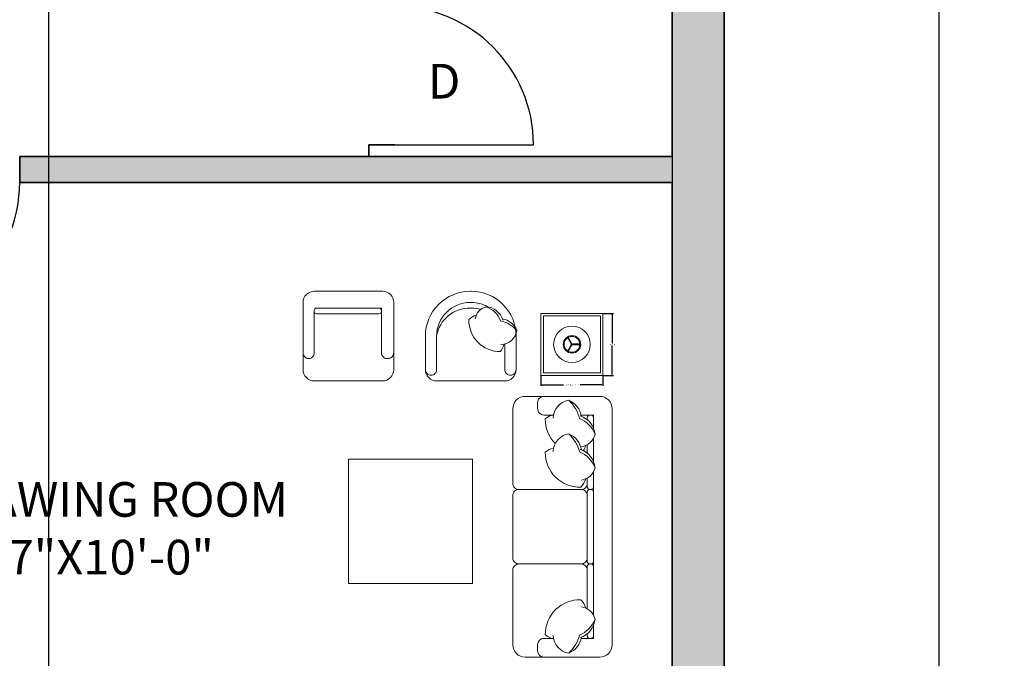
# Model space of a CAD drawing. Units: inches. Extents: x -5 to 330, y -522 to 40.
# Tile 19 of 23: x 159 to 330, y -380 to -269. Entities that reach past the tile are written whole.
import ezdxf

# ---------------------------------------------------------------- set-up
doc = ezdxf.new("R2010")
doc.units = ezdxf.units.IN
doc.header["$MEASUREMENT"] = 0
for name, color, linetype, lineweight in [('A-ANNO-DIMS', 2, 'Continuous', 18), ('A-ANNO-TEXT', 7, 'Continuous', 18), ('A-AREA-IDEN', 7, 'Continuous', 25), ('A-DOOR', 4, 'Continuous', 25), ('A-FURN', 8, 'Continuous', 18), ('A-WALL', 7, 'Continuous', 35)]:
    doc.layers.add(name, color=color, linetype=linetype, lineweight=lineweight)
doc.layers.add('A-WALL-PATT', color=18, linetype='Continuous', lineweight=13, true_color=0x000000)
doc.styles.get("Standard").update_dxf_attribs({"font": 'arial.ttf'})
doc.dimstyles.get("Standard").update_dxf_attribs({"dimtxt": 0.18, "dimasz": 0.18, "dimexe": 0.18, "dimexo": 0.0625, "dimgap": 0.09, "dimtad": 0, "dimtih": 1, "dimtoh": 1, "dimdec": 0, "dimzin": 0, "dimdsep": 46, "dimlunit": 3, "dimtxsty": 'Standard', "dimcen": 0.09, "dimadec": 0, "dimazin": 0, "dimtfac": 1, "dimtdec": 0, "dimtofl": 0, "dimtmove": 0, "dimatfit": 3, "dimfxl": 1, "dimtolj": 1, "dimtzin": 0, "dimarcsym": 0})

# ---------------------------------------------------------------- blocks, each defined once
blk = doc.blocks.new('*D6')
at = {"layer": 'A-ANNO-DIMS', "color": 0, "lineweight": -2, "transparency": 16777216}
for p, q in [((281.07, 12.36), (318.43, 12.36)), ((318.25, 12.18), (318.25, -238.29)), ((318.25, -494.96), (318.25, -244.5)), ((281.07, -495.14), (318.43, -495.14))]:
    blk.add_line(p, q, dxfattribs=at)
at = {"layer": 'A-ANNO-DIMS', "color": 0, "transparency": 16777216}
for points in [[(318.22, 12.18), (318.28, 12.18), (318.25, 12.36)], [(318.22, -494.96), (318.28, -494.96), (318.25, -495.14)]]:
    blk.add_solid(points, dxfattribs=at)
at = {"layer": 'Defpoints', "color": 0, "transparency": 16777216}
for p in [(281.01, 12.36), (281.01, -495.14), (318.25, -495.14)]:
    blk.add_point(p, dxfattribs=at)
at = {"layer": 'A-ANNO-DIMS', "color": 0, "transparency": 16777216, "insert": (318.25, -241.39), "char_height": 6, "attachment_point": 5}
blk.add_mtext('\\A1;42\'-4"', dxfattribs=at)
blk = doc.blocks.new('DOOR-24IN-SWING')
blk.add_line((24, 0), (24, 24))
blk.add_arc((24, 0), 24, 90, 180)
blk = doc.blocks.new('END-TABLE-SQUARE')
for p, q in [((5.32, 5.34), (4.56, 6.66)), ((5.32, 5.41), (4.56, 4.1)), ((5.44, 5.41), (4.68, 6.72)), ((5.44, 5.34), (4.68, 4.03)), ((5.38, 5.44), (6.89, 5.44)), ((5.38, 5.31), (6.89, 5.31))]:
    blk.add_line(p, q)
at = {"ltscale": 0.03}
blk.add_lwpolyline([(0, 0), (0, 10.75), (10.75, 10.75), (10.75, 0)], close=True, dxfattribs=at)
blk.add_lwpolyline([(0.43, 10.32), (0.43, 0.43), (10.32, 0.43), (10.32, 10.32)], close=True)
for radius in [3.17, 1.52, 1.36]:
    blk.add_circle((5.38, 5.38), radius)
blk = doc.blocks.new('*D27')
at = {"layer": 'A-ANNO-DIMS', "color": 0, "lineweight": -2, "transparency": 16777216}
for p, q in [((249.29, -330.63), (249.29, -332.36)), ((260.04, -330.63), (260.04, -332.36)), ((249.47, -332.18), (253.23, -332.18)), ((259.86, -332.18), (256.1, -332.18))]:
    blk.add_line(p, q, dxfattribs=at)
at = {"layer": 'A-ANNO-DIMS', "color": 0, "transparency": 16777216}
for points in [[(249.47, -332.15), (249.47, -332.21), (249.29, -332.18)], [(259.86, -332.15), (259.86, -332.21), (260.04, -332.18)]]:
    blk.add_solid(points, dxfattribs=at)
at = {"layer": 'Defpoints', "color": 0, "transparency": 16777216}
for p in [(249.29, -330.56), (260.04, -330.56), (260.04, -332.18)]:
    blk.add_point(p, dxfattribs=at)
at = {"layer": 'A-ANNO-DIMS', "color": 0, "transparency": 16777216, "insert": (254.67, -332.18), "char_height": 0.18, "attachment_point": 5}
blk.add_mtext('\\A1;END TABLE 0\'-11" TYP.', dxfattribs=at)
blk = doc.blocks.new('*D28')
at = {"layer": 'A-ANNO-DIMS', "color": 0, "lineweight": -2, "transparency": 16777216}
for p, q in [((260.11, -319.81), (261.84, -319.81)), ((261.66, -319.99), (261.66, -325)), ((261.66, -330.38), (261.66, -325.37)), ((260.11, -330.56), (261.84, -330.56))]:
    blk.add_line(p, q, dxfattribs=at)
at = {"layer": 'A-ANNO-DIMS', "color": 0, "transparency": 16777216}
for points in [[(261.63, -319.99), (261.69, -319.99), (261.66, -319.81)], [(261.63, -330.38), (261.69, -330.38), (261.66, -330.56)]]:
    blk.add_solid(points, dxfattribs=at)
at = {"layer": 'Defpoints', "color": 0, "transparency": 16777216}
for p in [(260.04, -319.81), (261.66, -319.81), (260.04, -330.56)]:
    blk.add_point(p, dxfattribs=at)
at = {"layer": 'A-ANNO-DIMS', "color": 0, "transparency": 16777216, "insert": (261.66, -325.19), "char_height": 0.18, "attachment_point": 5}
blk.add_mtext('\\A1;0\'-11" TYP.', dxfattribs=at)
blk = doc.blocks.new('*D37')
at = {"layer": 'A-ANNO-DIMS', "color": 0, "lineweight": -2, "transparency": 16777216}
for p, q in [((164.01, -53.21), (164.01, -522.31)), ((272.01, -53.21), (272.01, -522.31)), ((164.19, -522.13), (217.68, -522.13)), ((271.83, -522.13), (218.34, -522.13))]:
    blk.add_line(p, q, dxfattribs=at)
at = {"layer": 'A-ANNO-DIMS', "color": 0, "transparency": 16777216}
for points in [[(164.19, -522.1), (164.19, -522.16), (164.01, -522.13)], [(271.83, -522.1), (271.83, -522.16), (272.01, -522.13)]]:
    blk.add_solid(points, dxfattribs=at)
at = {"layer": 'Defpoints', "color": 0, "transparency": 16777216}
for p in [(164.01, -53.14), (272.01, -53.14), (272.01, -522.13)]:
    blk.add_point(p, dxfattribs=at)
at = {"layer": 'A-ANNO-DIMS', "color": 0, "transparency": 16777216, "insert": (218.01, -522.13), "char_height": 0.18, "attachment_point": 5}
blk.add_mtext('\\A1;9\'-0"', dxfattribs=at)

msp = doc.modelspace()

# ---------------------------------------------------------------- hatches: boundary and pattern name
at = {"layer": 'A-WALL-PATT'}
h = msp.add_hatch(color=256, dxfattribs=at)
h.dxf.hatch_style = 1
h.paths.add_polyline_path([(164.01, -44.15), (159.51, -44.15), (159.51, -153.14), (164.01, -153.14)], flags=17)
h.paths.add_polyline_path([(224.01, -188.14), (272.01, -188.14), (272.01, -218.14), (260.01, -218.14), (260.01, -222.64), (272.01, -222.64), (272.01, -292.64), (159.01, -292.64), (159.01, -297.14), (272.01, -297.14), (272.01, -417.14), (245.51, -417.14), (245.51, -426.14), (272.01, -426.14), (272.01, -495.14), (281.01, -495.14), (281.01, 12.36), (23.51, 12.36), (23.51, -426.14), (62.92, -426.14), (62.92, -417.14), (32.51, -417.14), (32.51, -297.14), (48.13, -297.14), (48.13, -292.64), (32.51, -292.64), (32.51, -140.64), (133.51, -140.64), (133.51, -131.64), (32.51, -131.64), (32.51, 3.36), (159.51, 3.36), (164.01, 3.36), (220.01, 3.36), (224.51, 3.36), (272.01, 3.36), (272.01, -179.14), (159.51, -179.14), (159.51, -188.14), (219.51, -188.14), (219.51, -266.64), (224.01, -266.64), (224.01, -222.64), (236.01, -222.64), (236.01, -218.14), (224.01, -218.14)])
h.paths.add_polyline_path([(133.01, -292.64), (128.51, -292.64), (128.51, -297.14), (128.51, -417.14), (122.92, -417.14), (122.92, -426.14), (133.01, -426.14)], flags=17)
h.paths.add_polyline_path([(185.51, -417.14), (159.01, -417.14), (159.01, -426.14), (185.51, -426.14)], flags=17)
h.paths.add_polyline_path([(133.51, -140.64), (129.01, -140.64), (129.01, -246.64), (133.51, -246.64)], flags=17)
h.paths.add_polyline_path([(246.01, -48.64), (224.51, -48.64), (224.51, -27.63), (220.01, -27.63), (220.01, -48.64), (198.6, -48.64), (198.6, -53.14), (246.01, -53.14)], flags=17)

# ---------------------------------------------------------------- linework, layer by layer
at = {"layer": 'A-FURN', "ltscale": 0.03}
for points in [[(210.04, -315.99), (210.04, -315.99, 0.414214), (208.1, -317.93), (208.1, -329.57, 0.414214), (210.04, -331.51), (210.04, -331.51), (221.87, -331.51, 0.414214), (223.8, -329.57), (223.8, -317.93, 0.414214), (221.87, -315.99)], [(246.57, -379.35, -0.414214), (244.42, -377.2), (244.42, -364.3, -0.414214), (245.5, -363.22, -0.414214), (244.42, -362.15), (244.42, -351.4, -0.414214), (245.5, -350.32, -0.414214), (244.42, -349.24), (244.42, -336.34, -0.414214), (246.57, -334.19), (259.48, -334.19, -0.414214), (261.63, -336.34), (261.63, -377.2, -0.414214), (259.48, -379.35)]]:
    msp.add_lwpolyline(points, format="xyb", close=True, dxfattribs=at)
msp.add_lwpolyline([(237.14, -331.51), (231.23, -331.51, -0.414214), (229.29, -329.57), (229.29, -323.75, -0.414214), (237.04, -315.99), (237.14, -315.99), (237.24, -315.99, -0.414214), (244.99, -323.75), (244.99, -329.57, -0.414214), (243.05, -331.51), (237.14, -331.51)], format="xyb", dxfattribs=at)
at = {"layer": 'A-FURN'}
for points in [[(218.02, -318.9), (210.42, -318.9, 0.414214), (210.04, -319.29), (210.04, -319.49, 0.414214), (210.42, -319.87), (217.04, -319.87, 0.414214)], [(217.04, -319.87), (221.28, -319.87, 0.414214), (221.67, -319.49), (221.67, -319.29, 0.414214), (221.28, -318.9)], [(221.28, -318.9), (218.02, -318.9, 0.414214)], [(231.23, -323.75, -0.414214), (237.04, -317.93), (237.14, -317.93)], [(231.23, -323.75, -0.372719), (237.04, -318.9), (237.14, -318.9)], [(240.12, -318.7, 0.130591), (237.24, -317.93), (237.14, -317.93)], [(238.89, -319.11, 0.072384), (237.24, -318.9), (237.14, -318.9)], [(242.71, -320.97, 0.306663), (239.82, -318.66, 0.30633), (237.93, -320.77, -0.872847)], [(245.15, -322.77, 0.14773), (242.32, -321.11, 0.213343), (239.82, -318.66, 0.178662)], [(210.04, -319.49), (210.04, -326.66, -0.414214), (209.07, -327.63), (209.07, -327.63, -0.414214), (208.1, -326.66)], [(242.86, -325.16, -0.165541), (242.26, -326.44, -0.425989), (236.82, -320.88, -0.121523), (238.11, -320.12, 7.115464)], [(242.37, -325.22, 0.356772), (245.15, -322.77, 0.249542), (242.63, -320.76, -9.61688)], [(231.23, -323.75), (231.23, -329.57, -0.414214), (230.26, -330.54), (230.26, -330.54, -0.414214), (229.29, -329.57)], [(223.8, -326.66, -0.414214), (222.83, -327.63), (222.64, -327.63, -0.414214), (221.67, -326.66), (221.67, -325.16)], [(243.05, -325.11), (243.05, -329.57, 0.414214), (244.02, -330.54), (244.02, -330.54, 0.414214), (244.99, -329.57)], [(251.47, -337.42), (249.8, -337.42, -0.414214), (248.72, -336.34), (248.72, -335.27, -0.414214), (249.8, -334.19)], [(251.4, -337.96, -0.356772), (254.11, -334.87, -0.249542), (256.34, -337.67, 9.61688)], [(254.11, -334.87, -0.14773), (255.96, -338.02, -0.213343), (258.67, -340.79, -0.178662)], [(251.47, -337.41, 0.165541), (250.04, -338.08, 0.200231), (251.78, -342.35, 0.121523)], [(256.11, -337.58, -0.306663), (258.67, -340.79, -0.30633), (256.33, -342.89, 0.872847)], [(258.4, -339.68), (258.4, -337.42), (256.29, -337.42, -0.414214)], [(257.33, -338.24), (257.33, -337.85, -0.414214), (257.76, -337.42), (257.97, -337.42, -0.414214), (258.4, -337.85)], [(258.4, -337.85), (258.4, -339.68, -0.414214)], [(251.4, -343.75, -0.356772), (254.11, -340.67, -0.249542), (256.34, -343.46, 9.61688)], [(254.11, -340.67, -0.14773), (255.96, -343.81, -0.213343), (258.67, -346.58, -0.178662)], [(256.63, -343.59, 0.071865), (257.05, -342.68, -7.115464)], [(257.33, -344.03), (257.33, -342.55, -0.414214)], [(258.4, -341.47), (258.4, -345.47, -0.414214)], [(251.47, -343.21, 0.165541), (250.04, -343.87, 0.425989), (256.2, -349.91, 0.121523), (257.05, -348.48, -7.115464)], [(256.11, -343.38, -0.306663), (258.67, -346.58, -0.30633), (256.33, -348.68, 0.872847)], [(258.4, -347.26), (258.4, -349.89, -0.414214), (257.97, -350.32), (257.76, -350.32, -0.414214), (257.33, -349.89), (257.33, -348.34, -0.414214)], [(257.33, -349.24, -0.414214), (256.25, -350.32), (245.5, -350.32, -0.414214)], [(257.33, -351.4, 0.414214), (256.25, -350.32)], [(257.33, -364.3, 0.414214), (256.25, -363.22), (245.5, -363.22, 0.414214)], [(257.33, -362.15, -0.414214), (256.25, -363.22)], [(258.4, -372.08), (258.4, -363.65, 0.414214), (257.97, -363.22), (257.76, -363.22, 0.414214), (257.33, -363.65), (257.33, -370.99, 0.414214)], [(251.47, -376.13, -0.165541), (250.04, -375.46, -0.425989), (256.2, -369.43, -0.121523), (257.05, -370.86, 7.115464)], [(256.11, -375.96, 0.306663), (258.67, -372.75, 0.30633), (256.33, -370.66, -0.872847)], [(254.11, -378.67, 0.14773), (255.96, -375.53, 0.213343), (258.67, -372.75, 0.178662)], [(258.4, -375.7), (258.4, -373.87, 0.414214)], [(249.8, -379.35, -0.414214), (248.72, -378.28), (248.72, -377.2, -0.414214), (249.8, -376.13), (251.47, -376.13)], [(251.4, -375.59, 0.356772), (254.11, -378.67, 0.249542), (256.34, -375.88, -9.61688)], [(257.33, -375.31), (257.33, -375.7, 0.414214), (257.76, -376.13), (257.97, -376.13, 0.414214), (258.4, -375.7)]]:
    msp.add_lwpolyline(points, format="xyb", dxfattribs=at)
for points in [[(218.02, -318.9), (210.13, -318.9)], [(221.67, -325.16), (221.67, -318.9), (218.02, -318.9)], [(258.4, -345.47), (258.4, -341.47)], [(258.4, -372.08), (258.4, -347.26)], [(256.29, -376.13), (258.4, -376.13), (258.4, -373.87)]]:
    msp.add_lwpolyline(points, dxfattribs=at)
at = {"layer": 'A-FURN', "ltscale": 0.03}
msp.add_lwpolyline([(215.96, -345.08), (215.96, -366.59), (237.46, -366.59), (237.46, -345.08)], close=True, dxfattribs=at)
at = {"layer": 'A-FURN'}
msp.add_lwpolyline([(258.4, -350.75), (258.4, -362.79, -0.414214), (257.97, -363.22), (257.76, -363.22, -0.414214), (257.33, -362.79), (257.33, -350.75, -0.414214), (257.76, -350.32), (257.97, -350.32, -0.414214)], format="xyb", close=True, dxfattribs=at)
at = {"layer": 'A-WALL'}
for p, q in [((281.01, 12.36), (281.01, -495.14)), ((272.01, -222.64), (272.01, -292.64)), ((219.51, -290.64), (224.01, -290.64)), ((219.51, -290.64), (219.51, -292.64)), ((159.01, -297.14), (159.01, -292.64)), ((159.01, -292.64), (272.01, -292.64)), ((159.01, -297.14), (272.01, -297.14)), ((272.01, -297.14), (272.01, -417.14))]:
    msp.add_line(p, q, dxfattribs=at)

# ---------------------------------------------------------------- block references
at = {"layer": 'A-DOOR'}
for p, rotation in [((224.01, -266.64), 269.9999999999999), ((159.01, -297.14), 180)]:
    msp.add_blockref('DOOR-24IN-SWING', p, dxfattribs=dict(at, rotation=rotation))
at = {"layer": 'A-FURN'}
msp.add_blockref('END-TABLE-SQUARE', (249.29, -330.56), dxfattribs=at)

# ---------------------------------------------------------------- texts
at = {"layer": 'A-ANNO-TEXT', "insert": (229.72, -276.61), "char_height": 6, "attachment_point": 1}
msp.add_mtext('D', dxfattribs=at)
at = {"layer": 'A-AREA-IDEN', "insert": (142.71, -349.04), "char_height": 6, "attachment_point": 1}
msp.add_mtext('DRAWING ROOM\\P11\'-7"X10\'-0"', dxfattribs=at)

# ---------------------------------------------------------------- dimensions: what is measured, and where the dimension line sits
at = {"layer": 'A-ANNO-DIMS'}
dim = msp.add_linear_dim(base=(318.24603734, -495.14358203), p1=(281.00988858, 12.35641797), p2=(281.00988858, -495.14358203), angle=90, dimstyle='Standard', override={"dimtxt": 6, "dimclrd": 0, "dimclre": 0, "dimclrt": 0}, dxfattribs=at)
dim.commit()
dim.dimension.update_dxf_attribs({"geometry": '*D6', "text_midpoint": (318.24603734, -241.39358203)})
dim = msp.add_linear_dim(base=(272.01, -522.13), p1=(164.01, -53.14), p2=(272.01, -53.14), dimstyle='Standard', override={"dimdec": 1, "dimlfac": 1, "dimrnd": 0, "dimzin": 1, "dimdsep": 46, "dimlunit": 4, "dimfrac": 2}, dxfattribs=at)
dim.commit()
dim.dimension.update_dxf_attribs({"geometry": '*D37', "text_midpoint": (218.01, -522.13)})
dim = msp.add_linear_dim(base=(261.6572, -319.8096), p1=(260.0442, -330.5629), p2=(260.0442, -319.8096), angle=90, text='<> TYP.', dimstyle='Standard', override={"dimdec": 1, "dimlfac": 1, "dimrnd": 0, "dimzin": 1, "dimdsep": 46, "dimlunit": 4, "dimfrac": 2}, dxfattribs=at)
dim.commit()
dim.dimension.update_dxf_attribs({"geometry": '*D28', "text_midpoint": (261.6572, -325.1863)})
dim = msp.add_linear_dim(base=(260.0442, -332.1759), p1=(249.2909, -330.5629), p2=(260.0442, -330.5629), text='END TABLE <> TYP.', dimstyle='Standard', override={"dimdec": 1, "dimlfac": 1, "dimrnd": 0, "dimzin": 1, "dimdsep": 46, "dimlunit": 4, "dimfrac": 2}, dxfattribs=at)
dim.commit()
dim.dimension.update_dxf_attribs({"geometry": '*D27', "text_midpoint": (254.6675, -332.1759)})

doc.saveas('drawing.dxf')
